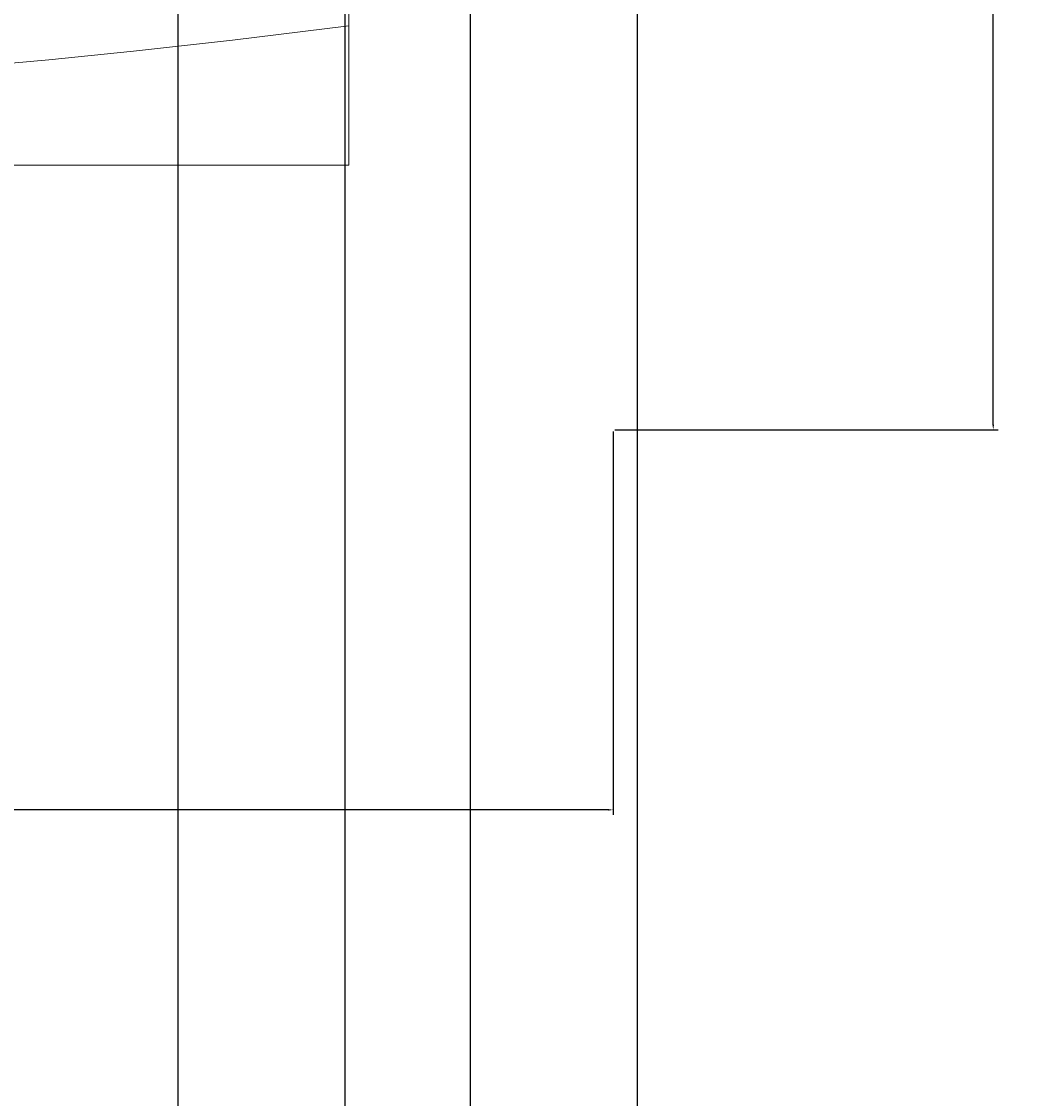
# Model space of a CAD drawing. Units: inches. Extents: x 7359 to 7979, y 33027 to 34263.
# Tile 8 of 32: x 7728 to 7764, y 33347 to 33386. Entities that reach past the tile are written whole.
import ezdxf

# ---------------------------------------------------------------- set-up
doc = ezdxf.new("R2010")
doc.units = ezdxf.units.IN
doc.layers.add('A-ANNO-DIMS', color=2, linetype='Continuous', lineweight=18)
doc.layers.add('A-FURN', color=8, linetype='Continuous', lineweight=18)
doc.styles.get("Standard").update_dxf_attribs({"font": 'arial.ttf'})
doc.dimstyles.get("Standard").update_dxf_attribs({"dimtxt": 0.18, "dimasz": 0.18, "dimexe": 0.18, "dimexo": 0.0625, "dimgap": 0.09, "dimtad": 0, "dimtih": 1, "dimtoh": 1, "dimdec": 4, "dimzin": 0, "dimdsep": 46, "dimtxsty": 'Standard', "dimcen": 0.09, "dimadec": 0, "dimazin": 0, "dimtfac": 1, "dimtdec": 4, "dimtofl": 0, "dimtmove": 0, "dimatfit": 3, "dimfxl": 1, "dimtolj": 1, "dimtzin": 0, "dimarcsym": 0})

# ---------------------------------------------------------------- blocks, each defined once
blk = doc.blocks.new('Dining Set - 36 x 72 in.')
for p, q in [((36, -18), (36, 18)), ((-36, -18), (36, -18))]:
    blk.add_line(p, q)
blk.add_lwpolyline([(22.6615, -14.44271), (25.2312, -14.21509), (28.2624, -13.9069), (31.8277, -13.50594), (36, -13)])
blk = doc.blocks.new('*D36')
at = {"layer": 'A-ANNO-DIMS', "color": 0, "lineweight": -2, "transparency": 16777216}
for p, q in [((7657.863, 33371.281), (7657.863, 33357.514)), ((7748.863, 33371.281), (7748.863, 33357.514)), ((7658.043, 33357.694), (7702.085, 33357.694)), ((7748.683, 33357.694), (7704.641, 33357.694))]:
    blk.add_line(p, q, dxfattribs=at)
at = {"layer": 'A-ANNO-DIMS', "color": 0, "transparency": 16777216}
for points in [[(7658.043, 33357.724), (7658.043, 33357.664), (7657.863, 33357.694)], [(7748.683, 33357.724), (7748.683, 33357.664), (7748.863, 33357.694)]]:
    blk.add_solid(points, dxfattribs=at)
at = {"layer": 'Defpoints', "color": 0, "transparency": 16777216}
for p in [(7657.863, 33371.344), (7748.863, 33371.344), (7748.863, 33357.694)]:
    blk.add_point(p, dxfattribs=at)
at = {"layer": 'A-ANNO-DIMS', "color": 0, "transparency": 16777216, "insert": (7703.363, 33357.694), "char_height": 0.18, "attachment_point": 5}
blk.add_mtext('\\A1;DINING SET 91 TYP.', dxfattribs=at)
blk = doc.blocks.new('*D37')
at = {"layer": 'A-ANNO-DIMS', "color": 0, "lineweight": -2, "transparency": 16777216}
for p, q in [((7748.925, 33426.344), (7762.693, 33426.344)), ((7762.513, 33426.164), (7762.513, 33399.025)), ((7762.513, 33371.524), (7762.513, 33398.662)), ((7748.925, 33371.344), (7762.693, 33371.344))]:
    blk.add_line(p, q, dxfattribs=at)
at = {"layer": 'A-ANNO-DIMS', "color": 0, "transparency": 16777216}
for points in [[(7762.483, 33426.164), (7762.543, 33426.164), (7762.513, 33426.344)], [(7762.483, 33371.524), (7762.543, 33371.524), (7762.513, 33371.344)]]:
    blk.add_solid(points, dxfattribs=at)
at = {"layer": 'Defpoints', "color": 0, "transparency": 16777216}
for p in [(7748.863, 33426.344), (7762.513, 33426.344), (7748.863, 33371.344)]:
    blk.add_point(p, dxfattribs=at)
at = {"layer": 'A-ANNO-DIMS', "color": 0, "transparency": 16777216, "insert": (7762.513, 33398.844), "char_height": 0.18, "attachment_point": 5}
blk.add_mtext('\\A1;55 TYP.', dxfattribs=at)
blk = doc.blocks.new('*D74')
at = {"layer": 'A-ANNO-DIMS', "color": 0, "lineweight": -2, "transparency": 16777216}
for p, q in [((7743.727, 33618.1), (7743.727, 33027.177)), ((7787.034, 33618.1), (7787.034, 33027.177)), ((7743.907, 33027.357), (7765, 33027.357)), ((7786.854, 33027.357), (7765.76, 33027.357))]:
    blk.add_line(p, q, dxfattribs=at)
at = {"layer": 'A-ANNO-DIMS', "color": 0, "transparency": 16777216}
for points in [[(7743.907, 33027.387), (7743.907, 33027.327), (7743.727, 33027.357)], [(7786.854, 33027.387), (7786.854, 33027.327), (7787.034, 33027.357)]]:
    blk.add_solid(points, dxfattribs=at)
at = {"layer": 'Defpoints', "color": 0, "transparency": 16777216}
for p in [(7743.727, 33618.162), (7787.034, 33618.162), (7787.034, 33027.357)]:
    blk.add_point(p, dxfattribs=at)
at = {"layer": 'A-ANNO-DIMS', "color": 0, "transparency": 16777216, "insert": (7765.38, 33027.357), "char_height": 0.18, "attachment_point": 5}
blk.add_mtext('\\A1;43.31', dxfattribs=at)
blk = doc.blocks.new('*D86')
at = {"layer": 'A-ANNO-DIMS', "color": 0, "lineweight": -2, "transparency": 16777216}
for p, q in [((7733.226578, 33475.599789), (7733.226578, 33027.176807)), ((7739.226578, 33475.599789), (7739.226578, 33027.176807)), ((7733.406578, 33027.356807), (7736.077151, 33027.356807)), ((7739.046578, 33027.356807), (7736.376005, 33027.356807))]:
    blk.add_line(p, q, dxfattribs=at)
at = {"layer": 'A-ANNO-DIMS', "color": 0, "transparency": 16777216}
for points in [[(7733.406578, 33027.386807), (7733.406578, 33027.326807), (7733.226578, 33027.356807)], [(7739.046578, 33027.386807), (7739.046578, 33027.326807), (7739.226578, 33027.356807)]]:
    blk.add_solid(points, dxfattribs=at)
at = {"layer": 'Defpoints', "color": 0, "transparency": 16777216}
for p in [(7733.226578, 33475.662289), (7739.226578, 33475.662289), (7739.226578, 33027.356807)]:
    blk.add_point(p, dxfattribs=at)
at = {"layer": 'A-ANNO-DIMS', "color": 0, "transparency": 16777216, "insert": (7736.226578, 33027.356807), "char_height": 0.18, "attachment_point": 5}
blk.add_mtext('\\A1;6', dxfattribs=at)
blk = doc.blocks.new('*D87')
at = {"layer": 'A-ANNO-DIMS', "color": 0, "lineweight": -2, "transparency": 16777216}
for p, q in [((7743.726578, 33453.099789), (7743.726578, 33027.176807)), ((7749.726578, 33453.099789), (7749.726578, 33027.176807)), ((7743.906578, 33027.356807), (7746.577151, 33027.356807)), ((7749.546578, 33027.356807), (7746.876005, 33027.356807))]:
    blk.add_line(p, q, dxfattribs=at)
at = {"layer": 'A-ANNO-DIMS', "color": 0, "transparency": 16777216}
for points in [[(7743.906578, 33027.386807), (7743.906578, 33027.326807), (7743.726578, 33027.356807)], [(7749.546578, 33027.386807), (7749.546578, 33027.326807), (7749.726578, 33027.356807)]]:
    blk.add_solid(points, dxfattribs=at)
at = {"layer": 'Defpoints', "color": 0, "transparency": 16777216}
for p in [(7743.726578, 33453.162289), (7749.726578, 33453.162289), (7749.726578, 33027.356807)]:
    blk.add_point(p, dxfattribs=at)
at = {"layer": 'A-ANNO-DIMS', "color": 0, "transparency": 16777216, "insert": (7746.726578, 33027.356807), "char_height": 0.18, "attachment_point": 5}
blk.add_mtext('\\A1;6', dxfattribs=at)

msp = doc.modelspace()

# ---------------------------------------------------------------- block references
at = {"layer": 'A-FURN'}
msp.add_blockref('Dining Set - 36 x 72 in.', (7703.363, 33398.8436), dxfattribs=at)

# ---------------------------------------------------------------- dimensions: what is measured, and where the dimension line sits
at = {"layer": 'A-ANNO-DIMS'}
for base, p1, p2, override, picture, middle in [((7787.0342, 33027.3568), (7743.7266, 33618.1623), (7787.0342, 33618.1623), {"dimdec": 2, "dimlfac": 1, "dimrnd": 0, "dimzin": 0, "dimdsep": 46, "dimlunit": 2}, '*D74', (7765.3804, 33027.3568)), ((7739.2266, 33027.3568), (7733.2266, 33475.6623), (7739.2266, 33475.6623), {"dimdec": 0, "dimlfac": 1, "dimrnd": 0, "dimzin": 0, "dimdsep": 46, "dimlunit": 2}, '*D86', (7736.2266, 33027.3568)), ((7749.7266, 33027.3568), (7743.7266, 33453.1623), (7749.7266, 33453.1623), {"dimdec": 0, "dimlfac": 1, "dimrnd": 0, "dimzin": 0, "dimdsep": 46, "dimlunit": 2}, '*D87', (7746.7266, 33027.3568))]:
    dim = msp.add_linear_dim(base=base, p1=p1, p2=p2, dimstyle='Standard', override=override, dxfattribs=at)
    dim.commit()
    dim.dimension.update_dxf_attribs({"geometry": picture, "text_midpoint": middle})
dim = msp.add_linear_dim(base=(7762.513, 33426.3436), p1=(7748.863, 33371.3436), p2=(7748.863, 33426.3436), angle=90, text='<> TYP.', dimstyle='Standard', override={"dimdec": 0, "dimlfac": 1, "dimrnd": 0, "dimzin": 0, "dimdsep": 46, "dimlunit": 2}, dxfattribs=at)
dim.commit()
dim.dimension.update_dxf_attribs({"geometry": '*D37', "text_midpoint": (7762.513, 33398.8436)})
dim = msp.add_linear_dim(base=(7748.863, 33357.6936), p1=(7657.863, 33371.3436), p2=(7748.863, 33371.3436), text='DINING SET <> TYP.', dimstyle='Standard', override={"dimdec": 0, "dimlfac": 1, "dimrnd": 0, "dimzin": 0, "dimdsep": 46, "dimlunit": 2}, dxfattribs=at)
dim.commit()
dim.dimension.update_dxf_attribs({"geometry": '*D36', "text_midpoint": (7703.363, 33357.6936)})

doc.saveas('drawing.dxf')
